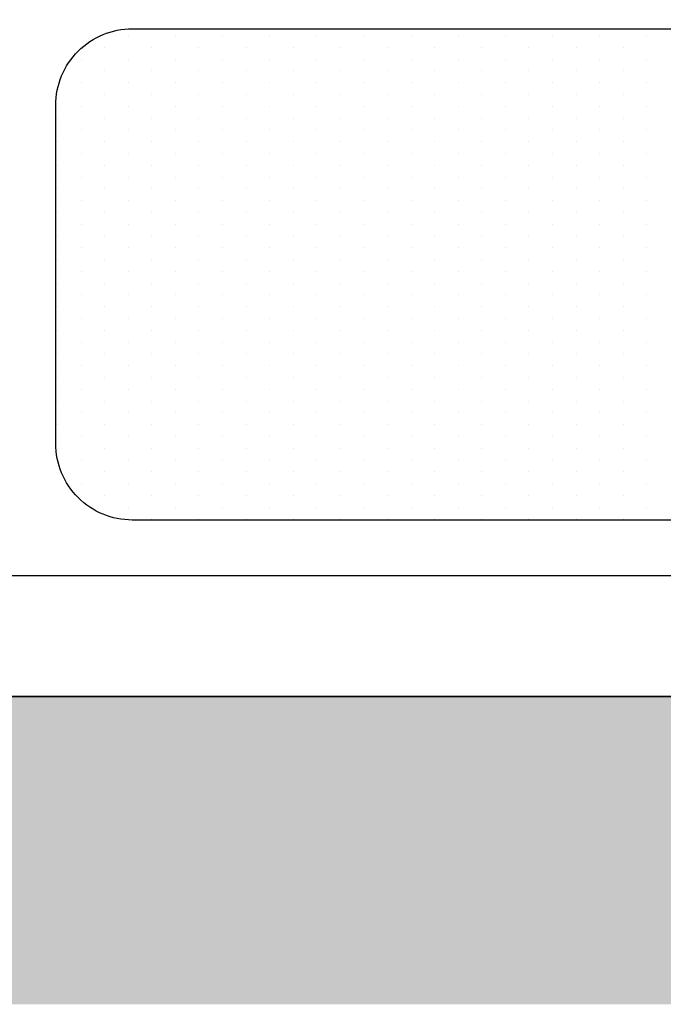
# Model space of a CAD drawing. Units: millimetres. Extents: x 2817 to 5038, y 1110 to 3565.
# Tile 4 of 21: x 2898 to 2917, y 1265 to 1294. Entities that reach past the tile are written whole.
import ezdxf

# ---------------------------------------------------------------- set-up
doc = ezdxf.new("R2010")
doc.units = ezdxf.units.MM
doc.layers.add('A-WALL', color=7, linetype='Continuous', lineweight=35)
doc.layers.add('FURNITURE', color=219, linetype='Continuous', lineweight=18)
doc.layers.add('A-WALL-PATT', color=51, linetype='Continuous', lineweight=13, true_color=0xf7f281)
doc.layers.add('BLOCK', color=6, linetype='Continuous')

# ---------------------------------------------------------------- blocks, each defined once
blk = doc.blocks.new('*X9')
at = {"color": 0}
for p, q in [((268.3125, 457.03125), (268.3125, 457.03125)), ((268.6875, 457.03125), (268.6875, 457.03125)), ((269.0625, 457.03125), (269.0625, 457.03125)), ((269.4375, 457.03125), (269.4375, 457.03125)), ((269.8125, 457.03125), (269.8125, 457.03125)), ((270.1875, 457.03125), (270.1875, 457.03125)), ((270.5625, 457.03125), (270.5625, 457.03125)), ((270.9375, 457.03125), (270.9375, 457.03125)), ((271.3125, 457.03125), (271.3125, 457.03125)), ((271.6875, 457.03125), (271.6875, 457.03125)), ((272.0625, 457.03125), (272.0625, 457.03125)), ((268.125, 456.9375), (268.125, 456.9375)), ((268.5, 456.9375), (268.5, 456.9375)), ((268.875, 456.9375), (268.875, 456.9375)), ((269.25, 456.9375), (269.25, 456.9375)), ((269.625, 456.9375), (269.625, 456.9375)), ((270, 456.9375), (270, 456.9375)), ((270.375, 456.9375), (270.375, 456.9375)), ((270.75, 456.9375), (270.75, 456.9375)), ((271.125, 456.9375), (271.125, 456.9375)), ((271.5, 456.9375), (271.5, 456.9375)), ((271.875, 456.9375), (271.875, 456.9375)), ((272.25, 456.9375), (272.25, 456.9375)), ((268.3125, 456.84375), (268.3125, 456.84375)), ((268.6875, 456.84375), (268.6875, 456.84375)), ((269.0625, 456.84375), (269.0625, 456.84375)), ((269.4375, 456.84375), (269.4375, 456.84375)), ((269.8125, 456.84375), (269.8125, 456.84375)), ((270.1875, 456.84375), (270.1875, 456.84375)), ((270.5625, 456.84375), (270.5625, 456.84375)), ((270.9375, 456.84375), (270.9375, 456.84375)), ((271.3125, 456.84375), (271.3125, 456.84375)), ((271.6875, 456.84375), (271.6875, 456.84375)), ((272.0625, 456.84375), (272.0625, 456.84375)), ((272.4375, 456.84375), (272.4375, 456.84375)), ((268.125, 456.75), (268.125, 456.75)), ((268.5, 456.75), (268.5, 456.75)), ((268.875, 456.75), (268.875, 456.75)), ((269.25, 456.75), (269.25, 456.75)), ((269.625, 456.75), (269.625, 456.75)), ((270, 456.75), (270, 456.75)), ((270.375, 456.75), (270.375, 456.75)), ((270.75, 456.75), (270.75, 456.75)), ((271.125, 456.75), (271.125, 456.75)), ((271.5, 456.75), (271.5, 456.75)), ((271.875, 456.75), (271.875, 456.75)), ((272.25, 456.75), (272.25, 456.75)), ((272.625, 456.75), (272.625, 456.75)), ((268.3125, 456.65625), (268.3125, 456.65625)), ((268.6875, 456.65625), (268.6875, 456.65625)), ((269.0625, 456.65625), (269.0625, 456.65625)), ((269.4375, 456.65625), (269.4375, 456.65625)), ((269.8125, 456.65625), (269.8125, 456.65625)), ((270.1875, 456.65625), (270.1875, 456.65625)), ((270.5625, 456.65625), (270.5625, 456.65625)), ((270.9375, 456.65625), (270.9375, 456.65625)), ((271.3125, 456.65625), (271.3125, 456.65625)), ((271.6875, 456.65625), (271.6875, 456.65625)), ((272.0625, 456.65625), (272.0625, 456.65625)), ((272.4375, 456.65625), (272.4375, 456.65625)), ((268.125, 456.5625), (268.125, 456.5625)), ((268.5, 456.5625), (268.5, 456.5625)), ((268.875, 456.5625), (268.875, 456.5625)), ((269.25, 456.5625), (269.25, 456.5625)), ((269.625, 456.5625), (269.625, 456.5625)), ((270, 456.5625), (270, 456.5625)), ((270.375, 456.5625), (270.375, 456.5625)), ((270.75, 456.5625), (270.75, 456.5625)), ((271.125, 456.5625), (271.125, 456.5625)), ((271.5, 456.5625), (271.5, 456.5625)), ((271.875, 456.5625), (271.875, 456.5625)), ((272.25, 456.5625), (272.25, 456.5625)), ((272.625, 456.5625), (272.625, 456.5625)), ((268.3125, 456.46875), (268.3125, 456.46875)), ((268.6875, 456.46875), (268.6875, 456.46875)), ((269.0625, 456.46875), (269.0625, 456.46875)), ((269.4375, 456.46875), (269.4375, 456.46875)), ((269.8125, 456.46875), (269.8125, 456.46875)), ((270.1875, 456.46875), (270.1875, 456.46875)), ((270.5625, 456.46875), (270.5625, 456.46875)), ((270.9375, 456.46875), (270.9375, 456.46875)), ((271.3125, 456.46875), (271.3125, 456.46875)), ((271.6875, 456.46875), (271.6875, 456.46875)), ((272.0625, 456.46875), (272.0625, 456.46875)), ((272.4375, 456.46875), (272.4375, 456.46875)), ((272.8125, 456.46875), (272.8125, 456.46875)), ((268.125, 456.375), (268.125, 456.375)), ((268.5, 456.375), (268.5, 456.375)), ((268.875, 456.375), (268.875, 456.375)), ((269.25, 456.375), (269.25, 456.375)), ((269.625, 456.375), (269.625, 456.375)), ((270, 456.375), (270, 456.375)), ((270.375, 456.375), (270.375, 456.375)), ((270.75, 456.375), (270.75, 456.375)), ((271.125, 456.375), (271.125, 456.375)), ((271.5, 456.375), (271.5, 456.375)), ((271.875, 456.375), (271.875, 456.375)), ((272.25, 456.375), (272.25, 456.375)), ((272.625, 456.375), (272.625, 456.375)), ((268.3125, 456.28125), (268.3125, 456.28125)), ((268.6875, 456.28125), (268.6875, 456.28125)), ((269.0625, 456.28125), (269.0625, 456.28125)), ((269.4375, 456.28125), (269.4375, 456.28125)), ((269.8125, 456.28125), (269.8125, 456.28125)), ((270.1875, 456.28125), (270.1875, 456.28125)), ((270.5625, 456.28125), (270.5625, 456.28125)), ((270.9375, 456.28125), (270.9375, 456.28125)), ((271.3125, 456.28125), (271.3125, 456.28125)), ((271.6875, 456.28125), (271.6875, 456.28125)), ((272.0625, 456.28125), (272.0625, 456.28125)), ((272.4375, 456.28125), (272.4375, 456.28125)), ((272.8125, 456.28125), (272.8125, 456.28125)), ((268.125, 456.1875), (268.125, 456.1875)), ((268.5, 456.1875), (268.5, 456.1875)), ((268.875, 456.1875), (268.875, 456.1875)), ((269.25, 456.1875), (269.25, 456.1875)), ((269.625, 456.1875), (269.625, 456.1875)), ((270, 456.1875), (270, 456.1875)), ((270.375, 456.1875), (270.375, 456.1875)), ((270.75, 456.1875), (270.75, 456.1875)), ((271.125, 456.1875), (271.125, 456.1875)), ((271.5, 456.1875), (271.5, 456.1875)), ((271.875, 456.1875), (271.875, 456.1875)), ((272.25, 456.1875), (272.25, 456.1875)), ((272.625, 456.1875), (272.625, 456.1875)), ((268.3125, 456.09375), (268.3125, 456.09375)), ((268.6875, 456.09375), (268.6875, 456.09375)), ((269.0625, 456.09375), (269.0625, 456.09375)), ((269.4375, 456.09375), (269.4375, 456.09375)), ((269.8125, 456.09375), (269.8125, 456.09375)), ((270.1875, 456.09375), (270.1875, 456.09375)), ((270.5625, 456.09375), (270.5625, 456.09375)), ((270.9375, 456.09375), (270.9375, 456.09375)), ((271.3125, 456.09375), (271.3125, 456.09375)), ((271.6875, 456.09375), (271.6875, 456.09375)), ((272.0625, 456.09375), (272.0625, 456.09375)), ((272.4375, 456.09375), (272.4375, 456.09375)), ((272.8125, 456.09375), (272.8125, 456.09375)), ((268.125, 456), (268.125, 456)), ((268.5, 456), (268.5, 456)), ((268.875, 456), (268.875, 456)), ((269.25, 456), (269.25, 456)), ((269.625, 456), (269.625, 456)), ((270, 456), (270, 456)), ((270.375, 456), (270.375, 456)), ((270.75, 456), (270.75, 456)), ((271.125, 456), (271.125, 456)), ((271.5, 456), (271.5, 456)), ((271.875, 456), (271.875, 456)), ((272.25, 456), (272.25, 456)), ((272.625, 456), (272.625, 456)), ((268.3125, 455.90625), (268.3125, 455.90625)), ((268.6875, 455.90625), (268.6875, 455.90625)), ((269.0625, 455.90625), (269.0625, 455.90625)), ((269.4375, 455.90625), (269.4375, 455.90625)), ((269.8125, 455.90625), (269.8125, 455.90625)), ((270.1875, 455.90625), (270.1875, 455.90625)), ((270.5625, 455.90625), (270.5625, 455.90625)), ((270.9375, 455.90625), (270.9375, 455.90625)), ((271.3125, 455.90625), (271.3125, 455.90625)), ((271.6875, 455.90625), (271.6875, 455.90625)), ((272.0625, 455.90625), (272.0625, 455.90625)), ((272.4375, 455.90625), (272.4375, 455.90625)), ((272.8125, 455.90625), (272.8125, 455.90625)), ((268.125, 455.8125), (268.125, 455.8125)), ((268.5, 455.8125), (268.5, 455.8125)), ((268.875, 455.8125), (268.875, 455.8125)), ((269.25, 455.8125), (269.25, 455.8125)), ((269.625, 455.8125), (269.625, 455.8125)), ((270, 455.8125), (270, 455.8125)), ((270.375, 455.8125), (270.375, 455.8125)), ((270.75, 455.8125), (270.75, 455.8125)), ((271.125, 455.8125), (271.125, 455.8125)), ((271.5, 455.8125), (271.5, 455.8125)), ((271.875, 455.8125), (271.875, 455.8125)), ((272.25, 455.8125), (272.25, 455.8125)), ((272.625, 455.8125), (272.625, 455.8125)), ((268.3125, 455.71875), (268.3125, 455.71875)), ((268.6875, 455.71875), (268.6875, 455.71875)), ((269.0625, 455.71875), (269.0625, 455.71875)), ((269.4375, 455.71875), (269.4375, 455.71875)), ((269.8125, 455.71875), (269.8125, 455.71875)), ((270.1875, 455.71875), (270.1875, 455.71875)), ((270.5625, 455.71875), (270.5625, 455.71875)), ((270.9375, 455.71875), (270.9375, 455.71875)), ((271.3125, 455.71875), (271.3125, 455.71875)), ((271.6875, 455.71875), (271.6875, 455.71875)), ((272.0625, 455.71875), (272.0625, 455.71875)), ((272.4375, 455.71875), (272.4375, 455.71875)), ((272.8125, 455.71875), (272.8125, 455.71875)), ((268.125, 455.625), (268.125, 455.625)), ((268.5, 455.625), (268.5, 455.625)), ((268.875, 455.625), (268.875, 455.625)), ((269.25, 455.625), (269.25, 455.625)), ((269.625, 455.625), (269.625, 455.625)), ((270, 455.625), (270, 455.625)), ((270.375, 455.625), (270.375, 455.625)), ((270.75, 455.625), (270.75, 455.625)), ((271.125, 455.625), (271.125, 455.625)), ((271.5, 455.625), (271.5, 455.625)), ((271.875, 455.625), (271.875, 455.625)), ((272.25, 455.625), (272.25, 455.625)), ((272.625, 455.625), (272.625, 455.625)), ((268.3125, 455.53125), (268.3125, 455.53125)), ((268.6875, 455.53125), (268.6875, 455.53125)), ((269.0625, 455.53125), (269.0625, 455.53125)), ((269.4375, 455.53125), (269.4375, 455.53125)), ((269.8125, 455.53125), (269.8125, 455.53125)), ((270.1875, 455.53125), (270.1875, 455.53125)), ((270.5625, 455.53125), (270.5625, 455.53125)), ((270.9375, 455.53125), (270.9375, 455.53125)), ((271.3125, 455.53125), (271.3125, 455.53125)), ((271.6875, 455.53125), (271.6875, 455.53125)), ((272.0625, 455.53125), (272.0625, 455.53125)), ((272.4375, 455.53125), (272.4375, 455.53125)), ((272.8125, 455.53125), (272.8125, 455.53125)), ((268.125, 455.4375), (268.125, 455.4375)), ((268.5, 455.4375), (268.5, 455.4375)), ((268.875, 455.4375), (268.875, 455.4375)), ((269.25, 455.4375), (269.25, 455.4375)), ((269.625, 455.4375), (269.625, 455.4375)), ((270, 455.4375), (270, 455.4375)), ((270.375, 455.4375), (270.375, 455.4375)), ((270.75, 455.4375), (270.75, 455.4375)), ((271.125, 455.4375), (271.125, 455.4375)), ((271.5, 455.4375), (271.5, 455.4375)), ((271.875, 455.4375), (271.875, 455.4375)), ((272.25, 455.4375), (272.25, 455.4375)), ((272.625, 455.4375), (272.625, 455.4375)), ((268.3125, 455.34375), (268.3125, 455.34375)), ((268.6875, 455.34375), (268.6875, 455.34375)), ((269.0625, 455.34375), (269.0625, 455.34375)), ((269.4375, 455.34375), (269.4375, 455.34375)), ((269.8125, 455.34375), (269.8125, 455.34375)), ((270.1875, 455.34375), (270.1875, 455.34375)), ((270.5625, 455.34375), (270.5625, 455.34375)), ((270.9375, 455.34375), (270.9375, 455.34375)), ((271.3125, 455.34375), (271.3125, 455.34375)), ((271.6875, 455.34375), (271.6875, 455.34375)), ((272.0625, 455.34375), (272.0625, 455.34375)), ((272.4375, 455.34375), (272.4375, 455.34375)), ((272.8125, 455.34375), (272.8125, 455.34375)), ((268.125, 455.25), (268.125, 455.25)), ((268.5, 455.25), (268.5, 455.25)), ((268.875, 455.25), (268.875, 455.25)), ((269.25, 455.25), (269.25, 455.25)), ((269.625, 455.25), (269.625, 455.25)), ((270, 455.25), (270, 455.25)), ((270.375, 455.25), (270.375, 455.25)), ((270.75, 455.25), (270.75, 455.25)), ((271.125, 455.25), (271.125, 455.25)), ((271.5, 455.25), (271.5, 455.25)), ((271.875, 455.25), (271.875, 455.25)), ((272.25, 455.25), (272.25, 455.25)), ((272.625, 455.25), (272.625, 455.25)), ((268.3125, 455.15625), (268.3125, 455.15625)), ((268.6875, 455.15625), (268.6875, 455.15625)), ((269.0625, 455.15625), (269.0625, 455.15625)), ((269.4375, 455.15625), (269.4375, 455.15625)), ((269.8125, 455.15625), (269.8125, 455.15625)), ((270.1875, 455.15625), (270.1875, 455.15625)), ((270.5625, 455.15625), (270.5625, 455.15625)), ((270.9375, 455.15625), (270.9375, 455.15625)), ((271.3125, 455.15625), (271.3125, 455.15625)), ((271.6875, 455.15625), (271.6875, 455.15625)), ((272.0625, 455.15625), (272.0625, 455.15625)), ((272.4375, 455.15625), (272.4375, 455.15625)), ((272.8125, 455.15625), (272.8125, 455.15625)), ((268.125, 455.0625), (268.125, 455.0625)), ((268.5, 455.0625), (268.5, 455.0625)), ((268.875, 455.0625), (268.875, 455.0625)), ((269.25, 455.0625), (269.25, 455.0625)), ((269.625, 455.0625), (269.625, 455.0625)), ((270, 455.0625), (270, 455.0625)), ((270.375, 455.0625), (270.375, 455.0625)), ((270.75, 455.0625), (270.75, 455.0625)), ((271.125, 455.0625), (271.125, 455.0625)), ((271.5, 455.0625), (271.5, 455.0625)), ((271.875, 455.0625), (271.875, 455.0625)), ((272.25, 455.0625), (272.25, 455.0625)), ((272.625, 455.0625), (272.625, 455.0625)), ((268.3125, 454.96875), (268.3125, 454.96875)), ((268.6875, 454.96875), (268.6875, 454.96875)), ((269.0625, 454.96875), (269.0625, 454.96875)), ((269.4375, 454.96875), (269.4375, 454.96875)), ((269.8125, 454.96875), (269.8125, 454.96875)), ((270.1875, 454.96875), (270.1875, 454.96875)), ((270.5625, 454.96875), (270.5625, 454.96875)), ((270.9375, 454.96875), (270.9375, 454.96875)), ((271.3125, 454.96875), (271.3125, 454.96875)), ((271.6875, 454.96875), (271.6875, 454.96875)), ((272.0625, 454.96875), (272.0625, 454.96875)), ((272.4375, 454.96875), (272.4375, 454.96875)), ((272.8125, 454.96875), (272.8125, 454.96875)), ((268.125, 454.875), (268.125, 454.875)), ((268.5, 454.875), (268.5, 454.875)), ((268.875, 454.875), (268.875, 454.875)), ((269.25, 454.875), (269.25, 454.875)), ((269.625, 454.875), (269.625, 454.875)), ((270, 454.875), (270, 454.875)), ((270.375, 454.875), (270.375, 454.875)), ((270.75, 454.875), (270.75, 454.875)), ((271.125, 454.875), (271.125, 454.875)), ((271.5, 454.875), (271.5, 454.875)), ((271.875, 454.875), (271.875, 454.875)), ((272.25, 454.875), (272.25, 454.875)), ((272.625, 454.875), (272.625, 454.875)), ((268.3125, 454.78125), (268.3125, 454.78125)), ((268.6875, 454.78125), (268.6875, 454.78125)), ((269.0625, 454.78125), (269.0625, 454.78125)), ((269.4375, 454.78125), (269.4375, 454.78125)), ((269.8125, 454.78125), (269.8125, 454.78125)), ((270.1875, 454.78125), (270.1875, 454.78125)), ((270.5625, 454.78125), (270.5625, 454.78125)), ((270.9375, 454.78125), (270.9375, 454.78125)), ((271.3125, 454.78125), (271.3125, 454.78125)), ((271.6875, 454.78125), (271.6875, 454.78125)), ((272.0625, 454.78125), (272.0625, 454.78125)), ((272.4375, 454.78125), (272.4375, 454.78125)), ((272.8125, 454.78125), (272.8125, 454.78125)), ((268.125, 454.6875), (268.125, 454.6875)), ((268.5, 454.6875), (268.5, 454.6875)), ((268.875, 454.6875), (268.875, 454.6875)), ((269.25, 454.6875), (269.25, 454.6875)), ((269.625, 454.6875), (269.625, 454.6875)), ((270, 454.6875), (270, 454.6875)), ((270.375, 454.6875), (270.375, 454.6875)), ((270.75, 454.6875), (270.75, 454.6875)), ((271.125, 454.6875), (271.125, 454.6875)), ((271.5, 454.6875), (271.5, 454.6875)), ((271.875, 454.6875), (271.875, 454.6875)), ((272.25, 454.6875), (272.25, 454.6875)), ((272.625, 454.6875), (272.625, 454.6875)), ((268.3125, 454.59375), (268.3125, 454.59375)), ((268.6875, 454.59375), (268.6875, 454.59375)), ((269.0625, 454.59375), (269.0625, 454.59375)), ((269.4375, 454.59375), (269.4375, 454.59375)), ((269.8125, 454.59375), (269.8125, 454.59375)), ((270.1875, 454.59375), (270.1875, 454.59375)), ((270.5625, 454.59375), (270.5625, 454.59375)), ((270.9375, 454.59375), (270.9375, 454.59375)), ((271.3125, 454.59375), (271.3125, 454.59375)), ((271.6875, 454.59375), (271.6875, 454.59375)), ((272.0625, 454.59375), (272.0625, 454.59375)), ((272.4375, 454.59375), (272.4375, 454.59375)), ((272.8125, 454.59375), (272.8125, 454.59375)), ((268.125, 454.5), (268.125, 454.5)), ((268.5, 454.5), (268.5, 454.5)), ((268.875, 454.5), (268.875, 454.5)), ((269.25, 454.5), (269.25, 454.5)), ((269.625, 454.5), (269.625, 454.5)), ((270, 454.5), (270, 454.5)), ((270.375, 454.5), (270.375, 454.5)), ((270.75, 454.5), (270.75, 454.5)), ((271.125, 454.5), (271.125, 454.5)), ((271.5, 454.5), (271.5, 454.5)), ((271.875, 454.5), (271.875, 454.5)), ((272.25, 454.5), (272.25, 454.5)), ((272.625, 454.5), (272.625, 454.5)), ((268.3125, 454.40625), (268.3125, 454.40625)), ((268.6875, 454.40625), (268.6875, 454.40625)), ((269.0625, 454.40625), (269.0625, 454.40625)), ((269.4375, 454.40625), (269.4375, 454.40625)), ((269.8125, 454.40625), (269.8125, 454.40625)), ((270.1875, 454.40625), (270.1875, 454.40625)), ((270.5625, 454.40625), (270.5625, 454.40625)), ((270.9375, 454.40625), (270.9375, 454.40625)), ((271.3125, 454.40625), (271.3125, 454.40625)), ((271.6875, 454.40625), (271.6875, 454.40625)), ((272.0625, 454.40625), (272.0625, 454.40625)), ((272.4375, 454.40625), (272.4375, 454.40625)), ((272.8125, 454.40625), (272.8125, 454.40625)), ((268.125, 454.3125), (268.125, 454.3125)), ((268.5, 454.3125), (268.5, 454.3125)), ((268.875, 454.3125), (268.875, 454.3125)), ((269.25, 454.3125), (269.25, 454.3125)), ((269.625, 454.3125), (269.625, 454.3125)), ((270, 454.3125), (270, 454.3125)), ((270.375, 454.3125), (270.375, 454.3125)), ((270.75, 454.3125), (270.75, 454.3125)), ((271.125, 454.3125), (271.125, 454.3125)), ((271.5, 454.3125), (271.5, 454.3125)), ((271.875, 454.3125), (271.875, 454.3125)), ((272.25, 454.3125), (272.25, 454.3125)), ((272.625, 454.3125), (272.625, 454.3125)), ((268.3125, 454.21875), (268.3125, 454.21875)), ((268.6875, 454.21875), (268.6875, 454.21875)), ((269.0625, 454.21875), (269.0625, 454.21875)), ((269.4375, 454.21875), (269.4375, 454.21875)), ((269.8125, 454.21875), (269.8125, 454.21875)), ((270.1875, 454.21875), (270.1875, 454.21875)), ((270.5625, 454.21875), (270.5625, 454.21875)), ((270.9375, 454.21875), (270.9375, 454.21875)), ((271.3125, 454.21875), (271.3125, 454.21875)), ((271.6875, 454.21875), (271.6875, 454.21875)), ((272.0625, 454.21875), (272.0625, 454.21875)), ((272.4375, 454.21875), (272.4375, 454.21875)), ((272.8125, 454.21875), (272.8125, 454.21875)), ((268.125, 454.125), (268.125, 454.125)), ((268.5, 454.125), (268.5, 454.125)), ((268.875, 454.125), (268.875, 454.125)), ((269.25, 454.125), (269.25, 454.125)), ((269.625, 454.125), (269.625, 454.125)), ((270, 454.125), (270, 454.125)), ((270.375, 454.125), (270.375, 454.125)), ((270.75, 454.125), (270.75, 454.125)), ((271.125, 454.125), (271.125, 454.125)), ((271.5, 454.125), (271.5, 454.125)), ((271.875, 454.125), (271.875, 454.125)), ((272.25, 454.125), (272.25, 454.125)), ((272.625, 454.125), (272.625, 454.125)), ((268.3125, 454.03125), (268.3125, 454.03125)), ((268.6875, 454.03125), (268.6875, 454.03125)), ((269.0625, 454.03125), (269.0625, 454.03125)), ((269.4375, 454.03125), (269.4375, 454.03125)), ((269.8125, 454.03125), (269.8125, 454.03125)), ((270.1875, 454.03125), (270.1875, 454.03125)), ((270.5625, 454.03125), (270.5625, 454.03125)), ((270.9375, 454.03125), (270.9375, 454.03125)), ((271.3125, 454.03125), (271.3125, 454.03125)), ((271.6875, 454.03125), (271.6875, 454.03125)), ((272.0625, 454.03125), (272.0625, 454.03125)), ((272.4375, 454.03125), (272.4375, 454.03125)), ((272.8125, 454.03125), (272.8125, 454.03125)), ((268.125, 453.9375), (268.125, 453.9375)), ((268.5, 453.9375), (268.5, 453.9375)), ((268.875, 453.9375), (268.875, 453.9375)), ((269.25, 453.9375), (269.25, 453.9375)), ((269.625, 453.9375), (269.625, 453.9375)), ((270, 453.9375), (270, 453.9375)), ((270.375, 453.9375), (270.375, 453.9375)), ((270.75, 453.9375), (270.75, 453.9375)), ((271.125, 453.9375), (271.125, 453.9375)), ((271.5, 453.9375), (271.5, 453.9375)), ((271.875, 453.9375), (271.875, 453.9375)), ((272.25, 453.9375), (272.25, 453.9375)), ((272.625, 453.9375), (272.625, 453.9375)), ((268.3125, 453.84375), (268.3125, 453.84375)), ((268.6875, 453.84375), (268.6875, 453.84375)), ((269.0625, 453.84375), (269.0625, 453.84375)), ((269.4375, 453.84375), (269.4375, 453.84375)), ((269.8125, 453.84375), (269.8125, 453.84375)), ((270.1875, 453.84375), (270.1875, 453.84375)), ((270.5625, 453.84375), (270.5625, 453.84375)), ((270.9375, 453.84375), (270.9375, 453.84375)), ((271.3125, 453.84375), (271.3125, 453.84375)), ((271.6875, 453.84375), (271.6875, 453.84375)), ((272.0625, 453.84375), (272.0625, 453.84375)), ((272.4375, 453.84375), (272.4375, 453.84375)), ((272.8125, 453.84375), (272.8125, 453.84375)), ((268.125, 453.75), (268.125, 453.75)), ((268.5, 453.75), (268.5, 453.75)), ((268.875, 453.75), (268.875, 453.75)), ((269.25, 453.75), (269.25, 453.75)), ((269.625, 453.75), (269.625, 453.75)), ((270, 453.75), (270, 453.75)), ((270.375, 453.75), (270.375, 453.75)), ((270.75, 453.75), (270.75, 453.75)), ((271.125, 453.75), (271.125, 453.75)), ((271.5, 453.75), (271.5, 453.75)), ((271.875, 453.75), (271.875, 453.75)), ((272.25, 453.75), (272.25, 453.75)), ((272.625, 453.75), (272.625, 453.75)), ((268.3125, 453.65625), (268.3125, 453.65625)), ((268.6875, 453.65625), (268.6875, 453.65625)), ((269.0625, 453.65625), (269.0625, 453.65625)), ((269.4375, 453.65625), (269.4375, 453.65625)), ((269.8125, 453.65625), (269.8125, 453.65625)), ((270.1875, 453.65625), (270.1875, 453.65625)), ((270.5625, 453.65625), (270.5625, 453.65625)), ((270.9375, 453.65625), (270.9375, 453.65625)), ((271.3125, 453.65625), (271.3125, 453.65625)), ((271.6875, 453.65625), (271.6875, 453.65625)), ((272.0625, 453.65625), (272.0625, 453.65625)), ((272.4375, 453.65625), (272.4375, 453.65625)), ((272.8125, 453.65625), (272.8125, 453.65625)), ((268.125, 453.5625), (268.125, 453.5625)), ((268.5, 453.5625), (268.5, 453.5625)), ((268.875, 453.5625), (268.875, 453.5625)), ((269.25, 453.5625), (269.25, 453.5625)), ((269.625, 453.5625), (269.625, 453.5625)), ((270, 453.5625), (270, 453.5625)), ((270.375, 453.5625), (270.375, 453.5625)), ((270.75, 453.5625), (270.75, 453.5625)), ((271.125, 453.5625), (271.125, 453.5625)), ((271.5, 453.5625), (271.5, 453.5625)), ((271.875, 453.5625), (271.875, 453.5625)), ((272.25, 453.5625), (272.25, 453.5625)), ((272.625, 453.5625), (272.625, 453.5625)), ((268.3125, 453.46875), (268.3125, 453.46875)), ((268.6875, 453.46875), (268.6875, 453.46875)), ((269.0625, 453.46875), (269.0625, 453.46875)), ((269.4375, 453.46875), (269.4375, 453.46875)), ((269.8125, 453.46875), (269.8125, 453.46875)), ((270.1875, 453.46875), (270.1875, 453.46875)), ((270.5625, 453.46875), (270.5625, 453.46875)), ((270.9375, 453.46875), (270.9375, 453.46875)), ((271.3125, 453.46875), (271.3125, 453.46875)), ((271.6875, 453.46875), (271.6875, 453.46875)), ((272.0625, 453.46875), (272.0625, 453.46875)), ((272.4375, 453.46875), (272.4375, 453.46875)), ((268.125, 453.375), (268.125, 453.375)), ((268.5, 453.375), (268.5, 453.375)), ((268.875, 453.375), (268.875, 453.375)), ((269.25, 453.375), (269.25, 453.375)), ((269.625, 453.375), (269.625, 453.375)), ((270, 453.375), (270, 453.375)), ((270.375, 453.375), (270.375, 453.375)), ((270.75, 453.375), (270.75, 453.375)), ((271.125, 453.375), (271.125, 453.375)), ((271.5, 453.375), (271.5, 453.375)), ((271.875, 453.375), (271.875, 453.375)), ((272.25, 453.375), (272.25, 453.375)), ((272.625, 453.375), (272.625, 453.375)), ((268.3125, 453.28125), (268.3125, 453.28125)), ((268.6875, 453.28125), (268.6875, 453.28125)), ((269.0625, 453.28125), (269.0625, 453.28125)), ((269.4375, 453.28125), (269.4375, 453.28125)), ((269.8125, 453.28125), (269.8125, 453.28125)), ((270.1875, 453.28125), (270.1875, 453.28125)), ((270.5625, 453.28125), (270.5625, 453.28125)), ((270.9375, 453.28125), (270.9375, 453.28125)), ((271.3125, 453.28125), (271.3125, 453.28125)), ((271.6875, 453.28125), (271.6875, 453.28125)), ((272.0625, 453.28125), (272.0625, 453.28125)), ((272.4375, 453.28125), (272.4375, 453.28125)), ((268.125, 453.1875), (268.125, 453.1875)), ((268.5, 453.1875), (268.5, 453.1875)), ((268.875, 453.1875), (268.875, 453.1875)), ((269.25, 453.1875), (269.25, 453.1875)), ((269.625, 453.1875), (269.625, 453.1875)), ((270, 453.1875), (270, 453.1875)), ((270.375, 453.1875), (270.375, 453.1875)), ((270.75, 453.1875), (270.75, 453.1875)), ((271.125, 453.1875), (271.125, 453.1875)), ((271.5, 453.1875), (271.5, 453.1875)), ((271.875, 453.1875), (271.875, 453.1875)), ((272.25, 453.1875), (272.25, 453.1875))]:
    blk.add_line(p, q, dxfattribs=at)
blk = doc.blocks.new('A$C52E67D0D')
at = {"layer": 'BLOCK'}
for points in [[(1901, 0), (601, 0, -0.414214), (501, 100), (501, 1700, -0.414214), (601, 1800), (1901, 1800, -0.414214), (2001, 1700), (2001, 100, -0.414214)], [(1171.77, 1365.08), (595.83, 1365.08, -0.414214), (534.98, 1425.93), (534.98, 1694.83, -0.414214), (595.83, 1755.67), (1171.77, 1755.67, -0.414214), (1232.61, 1694.83), (1232.61, 1425.93, -0.414214)]]:
    blk.add_lwpolyline(points, format="xyb", close=True, dxfattribs=at)
at = {"layer": 'BLOCK', "xscale": 100, "yscale": 100, "zscale": 100}
blk.add_blockref('*X9', (-26049.96, -43948.24), dxfattribs=at)

msp = doc.modelspace()

# ---------------------------------------------------------------- hatches: boundary and pattern name
at = {"layer": 'A-WALL-PATT'}
h = msp.add_hatch(color=256, dxfattribs=at)
h.dxf.hatch_style = 1
h.paths.add_polyline_path([(3186.7393, 1614.4357), (2841.7393, 1614.4357), (2841.7393, 1568.614), (2850.7393, 1568.7609), (2850.7393, 1605.4357), (2982.7393, 1605.4357), (2991.7393, 1605.4357), (3052.2393, 1605.4357), (3052.2393, 1573.7835), (3061.2393, 1573.7835), (3061.2393, 1605.4357), (3182.2393, 1605.4357), (3182.2393, 1143.4357), (3181.2393, 1143.4357), (3181.2393, 1134.4357), (3186.7393, 1134.4357)])
h.paths.add_polyline_path([(3061.2393, 1143.4357), (3061.2393, 1147.4357), (3052.2393, 1147.4357), (3052.2393, 1143.4357), (2850.7393, 1143.4357), (2850.7393, 1145.2996), (2841.7393, 1145.2996), (2841.7393, 1134.4357), (3061.2393, 1134.4357)], flags=17)
h.paths.add_polyline_path([(2850.7393, 1265.4357), (2946.7393, 1265.4357), (2946.7393, 1270.8357), (2946.7393, 1274.4357), (2850.7393, 1274.4357), (2850.7381, 1274.4357), (2850.7381, 1274.2564), (2841.7393, 1274.2564), (2841.7393, 1193.1527), (2850.7393, 1193.2996)], flags=17)
h.paths.add_polyline_path([(3061.2393, 1299.098), (3052.2393, 1299.098), (3052.2393, 1274.4357), (2991.7393, 1274.4357), (2991.7393, 1340.4357), (2982.7393, 1340.4357), (2982.7393, 1274.4357), (2982.7393, 1265.4357), (3052.2393, 1265.4357), (3052.2393, 1259.143), (3061.2393, 1259.2899)], flags=17)
h.paths.add_polyline_path([(3061.2393, 1383.4357), (3052.2393, 1383.4357), (3052.2393, 1379.4357), (2931.7393, 1379.4357), (2922.7393, 1379.4357), (2850.7393, 1379.4357), (2850.7381, 1379.4357), (2850.7381, 1379.3646), (2841.7393, 1379.3646), (2841.7393, 1322.1095), (2850.7393, 1322.2564), (2850.7393, 1370.4357), (2982.7393, 1370.4357), (2987.2393, 1370.4357), (3017.2393, 1370.4357), (3052.2393, 1370.4357), (3052.2393, 1323.098), (3061.2393, 1323.098)], flags=17)

# ---------------------------------------------------------------- linework, layer by layer
at = {"layer": 'A-WALL'}
msp.add_line((2850.7393, 1274.4357), (2946.7393, 1274.4357), dxfattribs=at)

# ---------------------------------------------------------------- block references
at = {"layer": 'FURNITURE', "xscale": 0.0367705835331598, "yscale": 0.0367705835331598, "zscale": 0.0367705835331598, "rotation": 180}
msp.add_blockref('A$C52E67D0D', (2944.6948, 1344.1495), dxfattribs=at)

doc.saveas('drawing.dxf')
